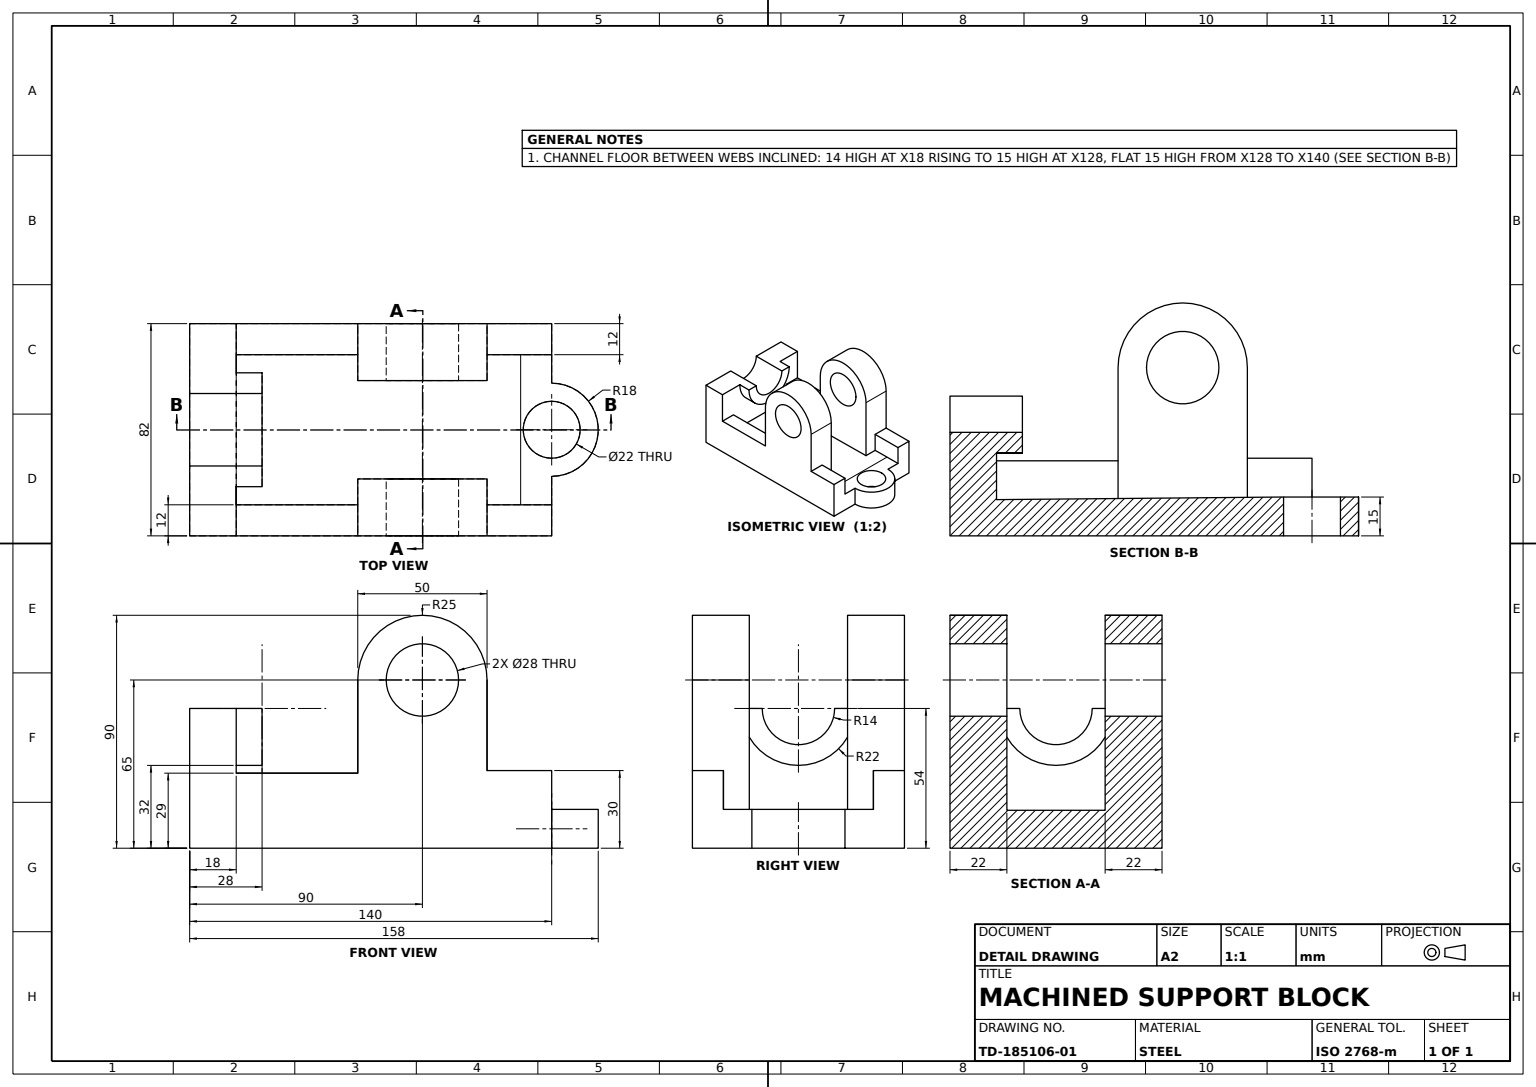
from build123d import *

# Parameters (mm, degrees)
BASE_BLOCK_DEPTH       = 82
POCKET_1_SKETCH_W      = 82
POCKET_1_SKETCH_H      = 15
POCKET_CUT_1_DEPTH     = 82
POCKET_2_SKETCH_W      = 12
POCKET_2_SKETCH_H      = 82
POCKET_CUT_2_DEPTH     = 82
PAD_SKETCH_W           = 12
PAD_SKETCH_H           = 15
FULL_WIDTH_PAD_DEPTH   = 82
LUG_1_DEPTH            = 22
LUG_START              = -22
LUG_2_DEPTH            = 22
WEB_1_DEPTH            = 12
WEB_2_DEPTH            = 12
WEB_3_DEPTH            = 12
WEB_4_DEPTH            = 12
LUG_BORE_SKETCH_R      = 14
LUG_BORE_DEPTH         = 100
EAR_BOSS_DEPTH         = 15
EAR_HOLE_SKETCH_R      = 11
EAR_HOLE_DEPTH         = 15
SIDE_BOSS_DEPTH        = 10
BEARING_SEAT_CUT_DEPTH = 28


with BuildPart() as part:
    # Base Profile Sketch → Base Block (new body)
    with BuildSketch(Plane.XY):
        Polygon((0, 15), (0, 0), (140, 0), (140, 30), (128, 30), (128, 15), (18, 14), (18, 54), (0, 54), align=None)
    extrude(amount=BASE_BLOCK_DEPTH)

    # Pocket 1 Sketch → Pocket Cut 1 (cut)
    with BuildSketch(Plane.ZY.offset(-128)):
        with Locations((41, 22.5)):
            Rectangle(POCKET_1_SKETCH_W, POCKET_1_SKETCH_H)
    extrude(amount=-POCKET_CUT_1_DEPTH, mode=Mode.SUBTRACT)

    # Pocket 2 Sketch → Pocket Cut 2 (cut)
    with BuildSketch(Plane(origin=(0, 15, 0), x_dir=(1, 0, 0), z_dir=(0, 1, 0))):
        with Locations((134, -41)):
            Rectangle(POCKET_2_SKETCH_W, POCKET_2_SKETCH_H)
    extrude(amount=-POCKET_CUT_2_DEPTH, mode=Mode.SUBTRACT)

    # Pad Sketch → Full Width Pad (add)
    with BuildSketch(Plane.XY.offset(82)):
        with Locations((134, 7.5)):
            Rectangle(PAD_SKETCH_W, PAD_SKETCH_H)
    extrude(amount=-FULL_WIDTH_PAD_DEPTH)

    # Lug 1 Sketch → Lug 1 (add)
    with BuildSketch(Plane.XY.offset(82)):
        with BuildLine():
            ThreePointArc((115, 65), (90, 90), (65, 65))
            Line((65, 65), (65, 14.427272727))
            Line((65, 14.427272727), (90, 14.654545455))
            Line((90, 14.654545455), (115, 14.881818182))
            Line((115, 14.881818182), (115, 65))
        make_face()
    extrude(amount=-LUG_1_DEPTH)

    # Lug 2 Sketch → Lug 2 (add)
    with BuildSketch(Plane(origin=(0, 0, 0), x_dir=(-1, 0, 0), z_dir=(0, 0, -1)).offset(LUG_START)):
        with BuildLine():
            Line((-115, 65), (-115, 14.881818182))
            Line((-115, 14.881818182), (-65, 14.427272727))
            Line((-65, 14.427272727), (-65, 65))
            ThreePointArc((-65, 65), (-90, 90), (-115, 65))
        make_face()
    extrude(amount=LUG_2_DEPTH)

    # Web 1 Sketch → Web 1 (add)
    with BuildSketch(Plane(origin=(0, 0, 0), x_dir=(-1, 0, 0), z_dir=(0, 0, -1))):
        Polygon((-18, 14), (-18, 29), (-65, 29), (-65, 14.427272727), align=None)
    extrude(amount=-WEB_1_DEPTH)

    # Web 2 Sketch → Web 2 (add)
    with BuildSketch(Plane(origin=(0, 0, 0), x_dir=(-1, 0, 0), z_dir=(0, 0, -1))):
        Polygon((-140, 15), (-140, 30), (-115, 30), (-115, 14.881818182), align=None)
    extrude(amount=-WEB_2_DEPTH)

    # Web 3 Sketch → Web 3 (add)
    with BuildSketch(Plane.XY.offset(82)):
        Polygon((115, 30), (115, 14.881818182), (140, 15), (140, 30), align=None)
    extrude(amount=-WEB_3_DEPTH)

    # Web 4 Sketch → Web 4 (add)
    with BuildSketch(Plane.XY.offset(82)):
        Polygon((18, 14), (18, 29), (65, 29), (65, 14.427272727), align=None)
    extrude(amount=-WEB_4_DEPTH)

    # Lug Bore Sketch → Lug Bore (cut)
    with BuildSketch(Plane.XY.offset(82)):
        with Locations((90, 65)):
            Circle(LUG_BORE_SKETCH_R)
    extrude(amount=-LUG_BORE_DEPTH, mode=Mode.SUBTRACT)

    # Ear Boss Sketch → Ear Boss (add)
    with BuildSketch(Plane(origin=(0, 15, 0), x_dir=(1, 0, 0), z_dir=(0, 1, 0))):
        with BuildLine():
            Line((140, -23), (140, -59))
            ThreePointArc((140, -59), (158, -41), (140, -23))
        make_face()
    extrude(amount=-EAR_BOSS_DEPTH)

    # Ear Hole Sketch → Ear Hole (cut)
    with BuildSketch(Plane(origin=(0, 15, 0), x_dir=(1, 0, 0), z_dir=(0, 1, 0))):
        with Locations(Location((140, -41, 0), (0, 0, 270))):
            Circle(EAR_HOLE_SKETCH_R)
    extrude(amount=-EAR_HOLE_DEPTH, mode=Mode.SUBTRACT)

    # Side Boss Sketch → Side Boss (add)
    with BuildSketch(Plane(origin=(18, 0, 0), x_dir=(0, 0, -1), z_dir=(1, 0, 0))):
        with BuildLine():
            Line((-63, 54), (-19, 54))
            ThreePointArc((-19, 54), (-41, 32), (-63, 54))
        make_face()
    extrude(amount=SIDE_BOSS_DEPTH)

    # Bearing Seat Sketch → Bearing Seat Cut (cut)
    with BuildSketch(Plane.ZY):
        with BuildLine():
            Line((27, 54), (55, 54))
            ThreePointArc((55, 54), (41, 40), (27, 54))
        make_face()
    extrude(amount=-BEARING_SEAT_CUT_DEPTH, mode=Mode.SUBTRACT)


solid = part.part
